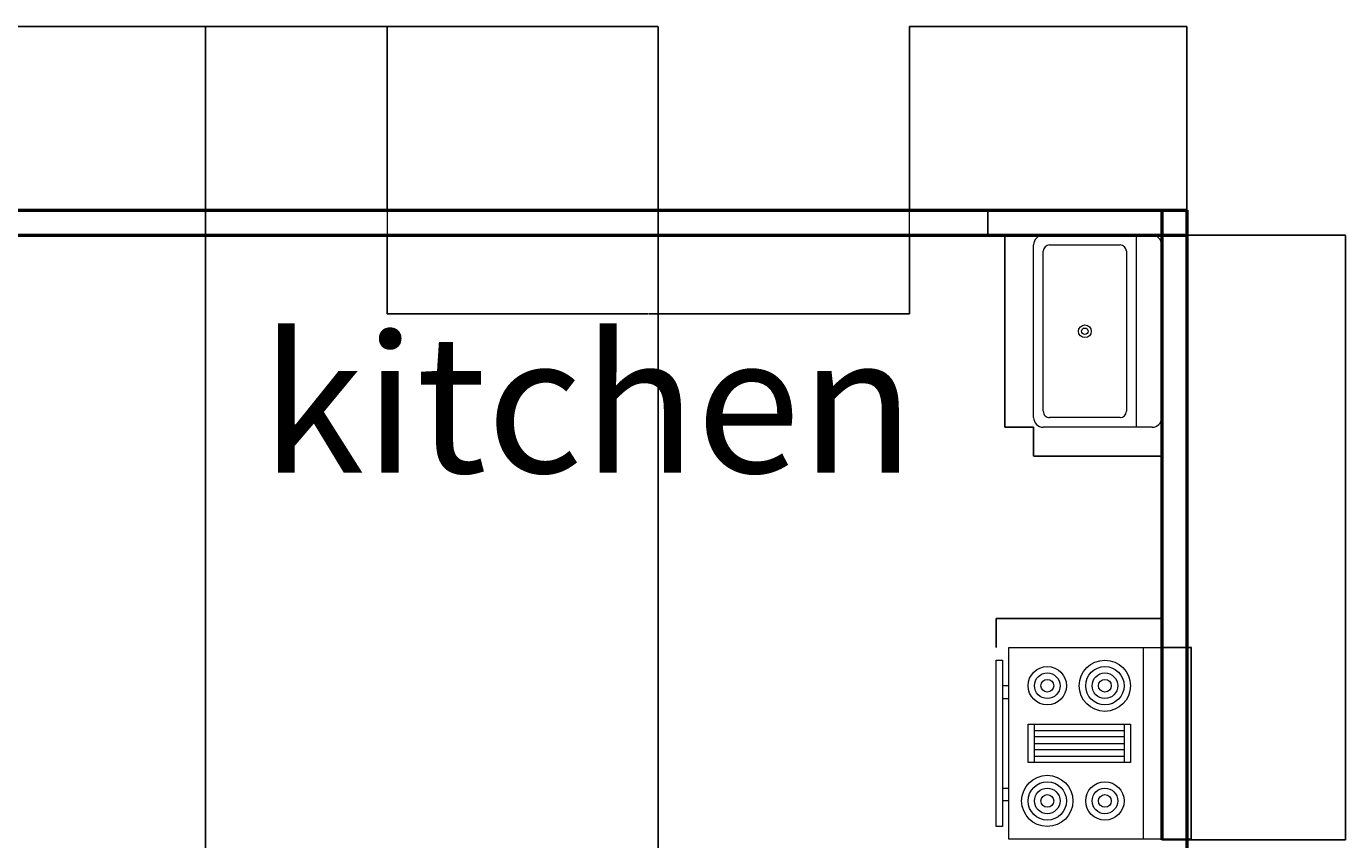
# Model space of a CAD drawing. Units: millimetres. Extents: x 756 to 17937, y 31 to 15590.
# Tile 5 of 6: x 7469 to 12704, y 12361 to 15590. Entities that reach past the tile are written whole.
import ezdxf

# ---------------------------------------------------------------- set-up
doc = ezdxf.new("R2010")
doc.units = ezdxf.units.MM
for name, color, linetype, lineweight in [('A-ANNO-DIMS', 2, 'Continuous', 18), ('A-AREA-IDEN', 7, 'Continuous', 25), ('A-EQPM', 8, 'Continuous', 18), ('A-FLOR-FIXT', 9, 'Continuous', 18), ('A-GLAZ', 4, 'Continuous', 18), ('A-WALL', 7, 'Continuous', 50)]:
    doc.layers.add(name, color=color, linetype=linetype, lineweight=lineweight)
doc.styles.get("Standard").update_dxf_attribs({"font": 'arial.ttf'})
doc.dimstyles.get("Standard").update_dxf_attribs({"dimtxt": 0.18, "dimasz": 0.18, "dimexe": 0.18, "dimexo": 0.0625, "dimgap": 0.09, "dimtad": 0, "dimtih": 1, "dimtoh": 1, "dimdec": 4, "dimzin": 0, "dimdsep": 46, "dimtxsty": 'Standard', "dimcen": 0.09, "dimadec": 0, "dimazin": 0, "dimtfac": 1, "dimtdec": 4, "dimtofl": 0, "dimtmove": 0, "dimatfit": 3, "dimfxl": 1, "dimtolj": 1, "dimtzin": 0, "dimarcsym": 0})

# ---------------------------------------------------------------- blocks, each defined once
blk = doc.blocks.new('Range-Oven - 30 in top')
for p, q in [((0, -3), (30, -3)), ((12, -6), (18, -6)), ((13, -20), (13, -6)), ((14, -6), (14, -20)), ((15, -20), (15, -6)), ((16, -6), (16, -20)), ((17, -20), (17, -6)), ((18, -20), (12, -20)), ((6, -24), (6, -25)), ((8, -25), (8, -24)), ((22, -25), (22, -24)), ((24, -24), (24, -25))]:
    blk.add_line(p, q)
for points in [[(0, -24), (0, 0), (30, 0), (30, -24)], [(12, -21), (12, -5), (18, -5), (18, -21)], [(2, -26), (2, -25), (28, -25), (28, -26)]]:
    blk.add_lwpolyline(points, close=True)
for centre, radius in [((6, -9), 4), ((6, -9), 3), ((24, -9), 3), ((6, -9), 2), ((6, -9), 1), ((24, -9), 2), ((24, -9), 1), ((24, -18), 4), ((6, -18), 3), ((6, -18), 2), ((24, -18), 3), ((24, -18), 2), ((6, -18), 1), ((24, -18), 1)]:
    blk.add_circle(centre, radius)
blk = doc.blocks.new('Sink-single - 30 in top')
blk.add_line((-15, -3.999996), (15, -3.999996))
for points in [[(-13.5, 0), (13.5, 0)], [(-15, -18.499996), (-15, -1.5)], [(15, -1.5), (15, -18.499996)], [(-12.5, -5.499996), (12.5, -5.499996)], [(-13.5, -17.499996), (-13.5, -6.499996)], [(13.5, -6.499996), (13.5, -17.499996)], [(12.5, -18.499996), (-12.5, -18.499996)], [(13.5, -19.999996), (-13.5, -19.999996)]]:
    blk.add_lwpolyline(points)
for radius in [1, 0.5]:
    blk.add_circle((0, -11.999996), radius)
for centre, radius, start, end in [((-13.5, -1.5), 1.5, 90, 180), ((13.5, -1.5), 1.5, 0, 90), ((-12.5, -6.499996), 1, 90, 180), ((12.5, -6.499996), 1, 0, 90), ((-13.5, -18.499996), 1.5, 180, 270), ((-12.5, -17.499996), 1, 180, 270), ((12.5, -17.499996), 1, 270, 0), ((13.5, -18.499996), 1.5, 270, 0)]:
    blk.add_arc(centre, radius, start, end)
blk = doc.blocks.new('WIN-2073')
for p, q in [((0, 100), (0, 0)), ((2072.9, 100), (0, 100)), ((2072.9, 0), (2072.9, 100)), ((0, 0), (2072.9, 0))]:
    blk.add_line(p, q)
blk = doc.blocks.new('*D17')
at = {"layer": 'A-ANNO-DIMS', "color": 0, "lineweight": -2, "transparency": 16777216}
for p, q in [((8900.8, 14760.1), (8900.8, 14449.1)), ((10973.7, 14760.1), (10973.7, 14449.1)), ((8900.9, 14449.2), (9935.9, 14449.2)), ((10973.5, 14449.2), (9938.5, 14449.2))]:
    blk.add_line(p, q, dxfattribs=at)
at = {"layer": 'A-ANNO-DIMS', "color": 0, "transparency": 16777216}
for points in [[(8900.9, 14449.3), (8900.9, 14449.2), (8900.8, 14449.2)], [(10973.5, 14449.3), (10973.5, 14449.2), (10973.7, 14449.2)]]:
    blk.add_solid(points, dxfattribs=at)
at = {"layer": 'Defpoints', "color": 0, "transparency": 16777216}
for p in [(8900.8, 14760.2), (10973.7, 14760.2), (10973.7, 14449.2)]:
    blk.add_point(p, dxfattribs=at)
at = {"layer": 'A-ANNO-DIMS', "color": 0, "transparency": 16777216, "insert": (9937.2, 14449.2), "char_height": 0.18, "attachment_point": 5}
blk.add_mtext('\\A1;WINDOW 2073 TYP.', dxfattribs=at)
blk = doc.blocks.new('*D18')
at = {"layer": 'A-ANNO-DIMS', "color": 0, "lineweight": -2, "transparency": 16777216}
for p, q in [((10973.7, 14860.2), (11284.8, 14860.2)), ((11284.6, 14860), (11284.6, 14810.4)), ((11284.6, 14760.4), (11284.6, 14810)), ((10973.7, 14760.2), (11284.8, 14760.2))]:
    blk.add_line(p, q, dxfattribs=at)
at = {"layer": 'A-ANNO-DIMS', "color": 0, "transparency": 16777216}
for points in [[(11284.6, 14860), (11284.6, 14860), (11284.6, 14860.2)], [(11284.6, 14760.4), (11284.6, 14760.4), (11284.6, 14760.2)]]:
    blk.add_solid(points, dxfattribs=at)
at = {"layer": 'Defpoints', "color": 0, "transparency": 16777216}
for p in [(10973.7, 14860.2), (11284.6, 14860.2), (10973.7, 14760.2)]:
    blk.add_point(p, dxfattribs=at)
at = {"layer": 'A-ANNO-DIMS', "color": 0, "transparency": 16777216, "insert": (11284.6, 14810.2), "char_height": 0.18, "attachment_point": 5}
blk.add_mtext('\\A1;100 TYP.', dxfattribs=at)
blk = doc.blocks.new('*D35')
at = {"layer": 'A-ANNO-DIMS', "color": 0, "lineweight": -2, "transparency": 16777216}
for p, q in [((11977.1, 13124.6), (12091.5, 13124.6)), ((12091.4, 13124.5), (12091.4, 12743.8)), ((12091.4, 12362.8), (12091.4, 12743.5)), ((11977.1, 12362.6), (12091.5, 12362.6))]:
    blk.add_line(p, q, dxfattribs=at)
at = {"layer": 'A-ANNO-DIMS', "color": 0, "transparency": 16777216}
for points in [[(12091.3, 13124.5), (12091.4, 13124.5), (12091.4, 13124.6)], [(12091.3, 12362.8), (12091.4, 12362.8), (12091.4, 12362.6)]]:
    blk.add_solid(points, dxfattribs=at)
at = {"layer": 'Defpoints', "color": 0, "transparency": 16777216}
for p in [(11977.1, 13124.6), (11977.1, 12362.6), (12091.4, 12362.6)]:
    blk.add_point(p, dxfattribs=at)
at = {"layer": 'A-ANNO-DIMS', "color": 0, "transparency": 16777216, "insert": (12091.4, 12743.6), "char_height": 0.18, "attachment_point": 5}
blk.add_mtext('\\A1;RANGE 762', dxfattribs=at)
blk = doc.blocks.new('*D36')
at = {"layer": 'A-ANNO-DIMS', "color": 0, "lineweight": -2, "transparency": 16777216}
for p, q in [((11316.7, 13124.7), (11316.7, 13239.1)), ((11316.8, 13238.9), (11646.6, 13238.9)), ((11976.9, 13238.9), (11647.1, 13238.9)), ((11977.1, 13124.7), (11977.1, 13239.1))]:
    blk.add_line(p, q, dxfattribs=at)
at = {"layer": 'A-ANNO-DIMS', "color": 0, "transparency": 16777216}
for points in [[(11316.8, 13239), (11316.8, 13238.9), (11316.7, 13238.9)], [(11976.9, 13239), (11976.9, 13238.9), (11977.1, 13238.9)]]:
    blk.add_solid(points, dxfattribs=at)
at = {"layer": 'Defpoints', "color": 0, "transparency": 16777216}
for p in [(11977.1, 13238.9), (11316.7, 13124.6), (11977.1, 13124.6)]:
    blk.add_point(p, dxfattribs=at)
at = {"layer": 'A-ANNO-DIMS', "color": 0, "transparency": 16777216, "insert": (11646.9, 13238.9), "char_height": 0.18, "attachment_point": 5}
blk.add_mtext('\\A1;660', dxfattribs=at)
blk = doc.blocks.new('*D37')
at = {"layer": 'A-ANNO-DIMS', "color": 0, "lineweight": -2, "transparency": 16777216}
for p, q in [((11465.7, 14760.4), (11351.3, 14760.4)), ((11351.5, 14760.2), (11351.5, 14379.5)), ((11351.5, 13998.5), (11351.5, 14379.2)), ((11465.7, 13998.4), (11351.3, 13998.4))]:
    blk.add_line(p, q, dxfattribs=at)
at = {"layer": 'A-ANNO-DIMS', "color": 0, "transparency": 16777216}
for points in [[(11351.5, 14760.2), (11351.5, 14760.2), (11351.5, 14760.4)], [(11351.5, 13998.5), (11351.5, 13998.5), (11351.5, 13998.4)]]:
    blk.add_solid(points, dxfattribs=at)
at = {"layer": 'Defpoints', "color": 0, "transparency": 16777216}
for p in [(11465.8, 14760.4), (11351.5, 13998.4), (11465.8, 13998.4)]:
    blk.add_point(p, dxfattribs=at)
at = {"layer": 'A-ANNO-DIMS', "color": 0, "transparency": 16777216, "insert": (11351.5, 14379.4), "char_height": 0.18, "attachment_point": 5}
blk.add_mtext('\\A1;SINK 762', dxfattribs=at)
blk = doc.blocks.new('*D38')
at = {"layer": 'A-ANNO-DIMS', "color": 0, "lineweight": -2, "transparency": 16777216}
for p, q in [((11465.8, 13998.3), (11465.8, 13883.9)), ((11973.8, 13998.3), (11973.8, 13883.9)), ((11466, 13884.1), (11719.5, 13884.1)), ((11973.6, 13884.1), (11720.1, 13884.1))]:
    blk.add_line(p, q, dxfattribs=at)
at = {"layer": 'A-ANNO-DIMS', "color": 0, "transparency": 16777216}
for points in [[(11466, 13884.1), (11466, 13884), (11465.8, 13884.1)], [(11973.6, 13884.1), (11973.6, 13884), (11973.8, 13884.1)]]:
    blk.add_solid(points, dxfattribs=at)
at = {"layer": 'Defpoints', "color": 0, "transparency": 16777216}
for p in [(11465.8, 13998.4), (11973.8, 13998.4), (11973.8, 13884.1)]:
    blk.add_point(p, dxfattribs=at)
at = {"layer": 'A-ANNO-DIMS', "color": 0, "transparency": 16777216, "insert": (11719.8, 13884.1), "char_height": 0.18, "attachment_point": 5}
blk.add_mtext('\\A1;508', dxfattribs=at)
blk = doc.blocks.new('*D52')
at = {"layer": 'A-ANNO-DIMS', "color": 0, "lineweight": -2, "transparency": 16777216}
for p, q in [((11974.2, 14760.2), (12703.5, 14760.2)), ((12703.4, 14760), (12703.4, 13560.4)), ((12703.4, 12360.4), (12703.4, 13560)), ((11974.2, 12360.2), (12703.5, 12360.2))]:
    blk.add_line(p, q, dxfattribs=at)
at = {"layer": 'A-ANNO-DIMS', "color": 0, "transparency": 16777216}
for points in [[(12703.3, 14760), (12703.4, 14760), (12703.4, 14760.2)], [(12703.3, 12360.4), (12703.4, 12360.4), (12703.4, 12360.2)]]:
    blk.add_solid(points, dxfattribs=at)
at = {"layer": 'Defpoints', "color": 0, "transparency": 16777216}
for p in [(11974.1, 14760.2), (11974.1, 12360.2), (12703.4, 12360.2)]:
    blk.add_point(p, dxfattribs=at)
at = {"layer": 'A-ANNO-DIMS', "color": 0, "transparency": 16777216, "insert": (12703.4, 13560.2), "char_height": 0.18, "attachment_point": 5}
blk.add_mtext('\\A1;2400', dxfattribs=at)
blk = doc.blocks.new('*D55')
at = {"layer": 'A-ANNO-DIMS', "color": 0, "lineweight": -2, "transparency": 16777216}
for p, q in [((6374.1, 14860.2), (6374.1, 15589.6)), ((6374.3, 15589.4), (7637, 15589.4)), ((8900.6, 15589.4), (7637.9, 15589.4)), ((8900.8, 14860.2), (8900.8, 15589.6))]:
    blk.add_line(p, q, dxfattribs=at)
at = {"layer": 'A-ANNO-DIMS', "color": 0, "transparency": 16777216}
for points in [[(6374.3, 15589.5), (6374.3, 15589.4), (6374.1, 15589.4)], [(8900.6, 15589.5), (8900.6, 15589.4), (8900.8, 15589.4)]]:
    blk.add_solid(points, dxfattribs=at)
at = {"layer": 'Defpoints', "color": 0, "transparency": 16777216}
for p in [(8900.8, 15589.4), (6374.1, 14860.2), (8900.8, 14860.2)]:
    blk.add_point(p, dxfattribs=at)
at = {"layer": 'A-ANNO-DIMS', "color": 0, "transparency": 16777216, "insert": (7637.4, 15589.4), "char_height": 0.18, "attachment_point": 5}
blk.add_mtext('\\A1;2526.6', dxfattribs=at)
blk = doc.blocks.new('*D56')
at = {"layer": 'A-ANNO-DIMS', "color": 0, "lineweight": -2, "transparency": 16777216}
for p, q in [((10973.7, 14860.2), (10973.7, 15589.6)), ((10973.8, 15589.4), (11523.4, 15589.4)), ((12073.9, 15589.4), (11524.3, 15589.4)), ((12074.1, 14860.2), (12074.1, 15589.6))]:
    blk.add_line(p, q, dxfattribs=at)
at = {"layer": 'A-ANNO-DIMS', "color": 0, "transparency": 16777216}
for points in [[(10973.8, 15589.5), (10973.8, 15589.4), (10973.7, 15589.4)], [(12073.9, 15589.5), (12073.9, 15589.4), (12074.1, 15589.4)]]:
    blk.add_solid(points, dxfattribs=at)
at = {"layer": 'Defpoints', "color": 0, "transparency": 16777216}
for p in [(12074.1, 15589.4), (10973.7, 14860.2), (12074.1, 14860.2)]:
    blk.add_point(p, dxfattribs=at)
at = {"layer": 'A-ANNO-DIMS', "color": 0, "transparency": 16777216, "insert": (11523.9, 15589.4), "char_height": 0.18, "attachment_point": 5}
blk.add_mtext('\\A1;1100.5', dxfattribs=at)
blk = doc.blocks.new('*D61')
at = {"layer": 'A-ANNO-DIMS', "color": 0, "lineweight": -2, "transparency": 16777216}
for p, q in [((8180.2, 7660.2), (8180.2, 15589.6)), ((8180.4, 15589.4), (9077.5, 15589.4)), ((9975.2, 15589.4), (9078.2, 15589.4)), ((9975.4, 7660.2), (9975.4, 15589.6))]:
    blk.add_line(p, q, dxfattribs=at)
at = {"layer": 'A-ANNO-DIMS', "color": 0, "transparency": 16777216}
for points in [[(8180.4, 15589.5), (8180.4, 15589.4), (8180.2, 15589.4)], [(9975.2, 15589.5), (9975.2, 15589.4), (9975.4, 15589.4)]]:
    blk.add_solid(points, dxfattribs=at)
at = {"layer": 'Defpoints', "color": 0, "transparency": 16777216}
for p in [(9975.4, 15589.4), (8180.2, 7660.2), (9975.4, 7660.2)]:
    blk.add_point(p, dxfattribs=at)
at = {"layer": 'A-ANNO-DIMS', "color": 0, "transparency": 16777216, "insert": (9077.8, 15589.4), "char_height": 0.18, "attachment_point": 5}
blk.add_mtext('\\A1;1795', dxfattribs=at)

msp = doc.modelspace()

# ---------------------------------------------------------------- linework, layer by layer
at = {"layer": 'A-WALL'}
for p, q in [((6374.114, 14860.181), (11974.114, 14860.181)), ((11974.114, 14860.181), (11974.114, 12360.181)), ((11974.114, 14860.181), (12074.114, 14860.181)), ((12074.114, 14860.181), (12074.114, 14737.835)), ((6274.114, 14760.181), (11974.114, 14760.181)), ((11974.114, 14760.181), (12074.114, 14760.181)), ((12074.114, 14760.181), (12074.114, 7560.16))]:
    msp.add_line(p, q, dxfattribs=at)

# ---------------------------------------------------------------- block references
at = {"layer": 'A-EQPM', "xscale": 25.4, "yscale": 25.4, "zscale": 25.4, "rotation": 270}
msp.add_blockref('Range-Oven - 30 in top', (11977.056, 13124.644), dxfattribs=at)
at = {"layer": 'A-FLOR-FIXT', "xscale": 25.4, "yscale": 25.4, "zscale": 25.4, "rotation": 270}
msp.add_blockref('Sink-single - 30 in top', (11973.81, 14379.363), dxfattribs=at)
at = {"layer": 'A-GLAZ'}
msp.add_blockref('WIN-2073', (8900.754, 14760.181), dxfattribs=at)

# ---------------------------------------------------------------- texts
at = {"layer": 'A-AREA-IDEN', "insert": (8398.561, 14363.696), "char_height": 545.7898, "attachment_point": 1}
msp.add_mtext_dynamic_manual_height_columns('kitchen', width=18937.89877, gutter_width=34.112, heights=[0], dxfattribs=at)

# ---------------------------------------------------------------- dimensions: what is measured, and where the dimension line sits
at = {"layer": 'A-ANNO-DIMS'}
for base, p1, p2, override, picture, middle in [((8900.754, 15589.431), (6374.114, 14860.181), (8900.754, 14860.181), {"dimdec": 1, "dimlfac": 1, "dimrnd": 0, "dimzin": 0, "dimdsep": 46, "dimlunit": 2}, '*D55', (7637.434, 15589.431)), ((9975.382, 15589.431), (8180.23, 7660.181), (9975.382, 7660.181), {"dimdec": 0, "dimlfac": 1, "dimrnd": 0, "dimzin": 0, "dimdsep": 46, "dimlunit": 2}, '*D61', (9077.806, 15589.431)), ((12074.114, 15589.431), (10973.658, 14860.181), (12074.114, 14860.181), {"dimdec": 1, "dimlfac": 1, "dimrnd": 0, "dimzin": 0, "dimdsep": 46, "dimlunit": 2}, '*D56', (11523.886, 15589.431)), ((11973.81, 13884.063), (11465.811, 13998.363), (11973.81, 13998.363), {"dimdec": 0, "dimlfac": 1, "dimrnd": 0, "dimzin": 0, "dimdsep": 46, "dimlunit": 2}, '*D38', (11719.81, 13884.063)), ((11977.056, 13238.944), (11316.657, 13124.644), (11977.056, 13124.644), {"dimdec": 0, "dimlfac": 1, "dimrnd": 0, "dimzin": 0, "dimdsep": 46, "dimlunit": 2}, '*D36', (11646.857, 13238.944))]:
    dim = msp.add_linear_dim(base=base, p1=p1, p2=p2, dimstyle='Standard', override=override, dxfattribs=at)
    dim.commit()
    dim.dimension.update_dxf_attribs({"geometry": picture, "text_midpoint": middle})
for base, p1, p2, angle, text, picture, middle in [((11284.593, 14860.181), (10973.658, 14760.181), (10973.658, 14860.181), 90, '<> TYP.', '*D18', (11284.593, 14810.181)), ((11351.511, 13998.363), (11465.811, 14760.363), (11465.811, 13998.363), 270, 'SINK <>', '*D37', (11351.511, 14379.363)), ((12091.356, 12362.644), (11977.056, 13124.644), (11977.056, 12362.644), 270, 'RANGE <>', '*D35', (12091.356, 12743.644))]:
    dim = msp.add_linear_dim(base=base, p1=p1, p2=p2, angle=angle, text=text, dimstyle='Standard', override={"dimdec": 0, "dimlfac": 1, "dimrnd": 0, "dimzin": 0, "dimdsep": 46, "dimlunit": 2}, dxfattribs=at)
    dim.commit()
    dim.dimension.update_dxf_attribs({"geometry": picture, "text_midpoint": middle})
dim = msp.add_linear_dim(base=(10973.658, 14449.245), p1=(8900.754, 14760.181), p2=(10973.658, 14760.181), text='WINDOW <> TYP.', dimstyle='Standard', override={"dimdec": 0, "dimlfac": 1, "dimrnd": 0, "dimzin": 0, "dimdsep": 46, "dimlunit": 2}, dxfattribs=at)
dim.commit()
dim.dimension.update_dxf_attribs({"geometry": '*D17', "text_midpoint": (9937.206, 14449.245)})
dim = msp.add_linear_dim(base=(12703.364, 12360.181), p1=(11974.114, 14760.181), p2=(11974.114, 12360.181), angle=270, dimstyle='Standard', override={"dimdec": 0, "dimlfac": 1, "dimrnd": 0, "dimzin": 0, "dimdsep": 46, "dimlunit": 2}, dxfattribs=at)
dim.commit()
dim.dimension.update_dxf_attribs({"geometry": '*D52', "text_midpoint": (12703.364, 13560.181)})

doc.saveas('drawing.dxf')
